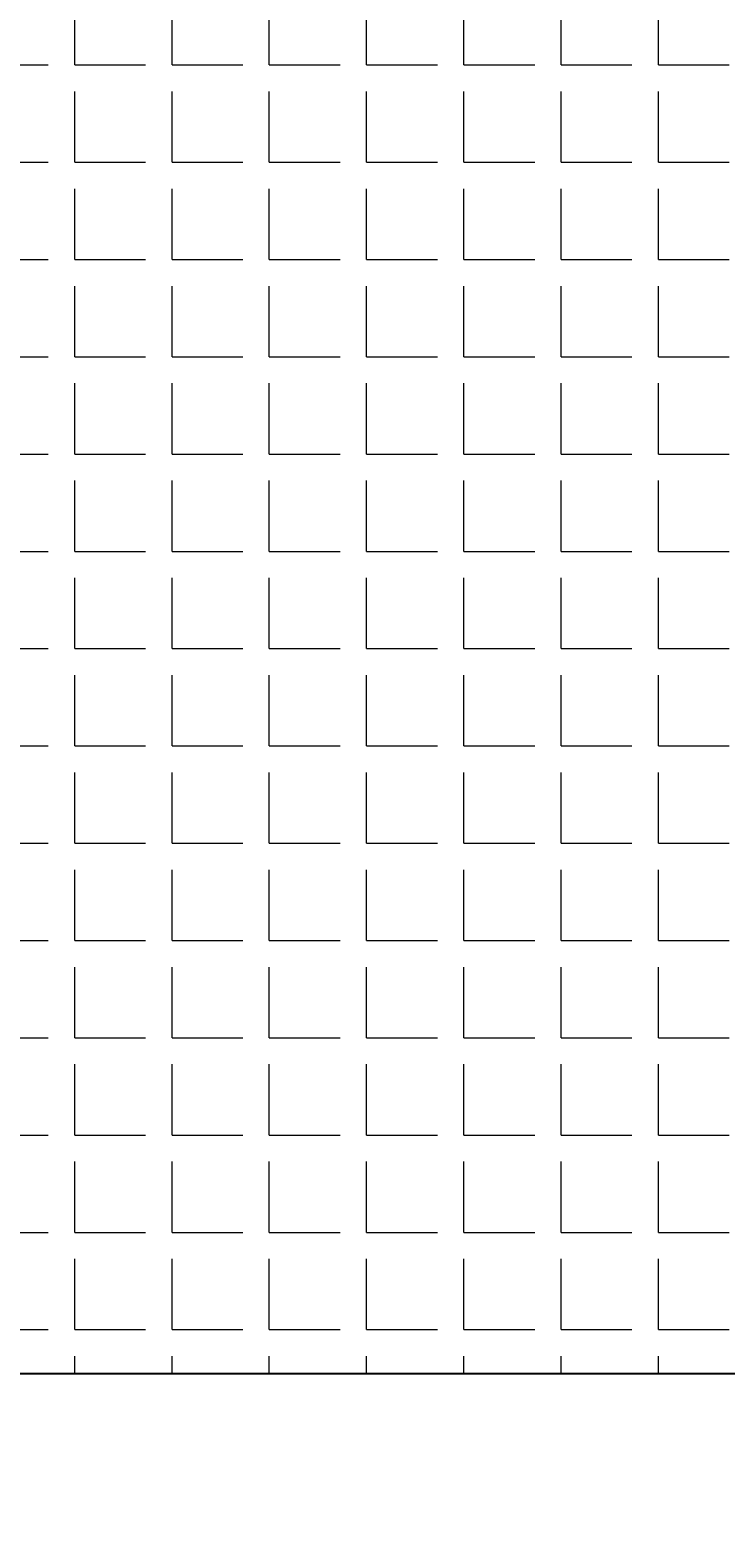
# Model space of a CAD drawing. Units: inches. Extents: x 84 to 1044, y -280 to 906.
# Tile 13 of 105: x 521 to 571, y -132 to -25. Entities that reach past the tile are written whole.
import ezdxf

# ---------------------------------------------------------------- set-up
doc = ezdxf.new("R2010")
doc.units = ezdxf.units.IN
doc.layers.add('A-ANNO-DIMS', color=2, linetype='Continuous', lineweight=18)
doc.layers.add('C-PROP', color=7, linetype='Continuous', lineweight=25)
doc.layers.add('L-HRDS-PATT', color=23, linetype='Continuous', lineweight=9, true_color=0xc2877b)
doc.styles.get("Standard").update_dxf_attribs({"font": 'arial.ttf'})
doc.dimstyles.get("Standard").update_dxf_attribs({"dimtxt": 0.18, "dimasz": 0.18, "dimexe": 0.18, "dimexo": 0.0625, "dimgap": 0.09, "dimtad": 0, "dimtih": 1, "dimtoh": 1, "dimdec": 4, "dimzin": 0, "dimdsep": 46, "dimtxsty": 'Standard', "dimcen": 0.09, "dimadec": 0, "dimazin": 0, "dimtfac": 1, "dimtdec": 4, "dimtofl": 0, "dimtmove": 0, "dimatfit": 3, "dimfxl": 1, "dimtolj": 1, "dimtzin": 0, "dimarcsym": 0})

# ---------------------------------------------------------------- blocks, each defined once
blk = doc.blocks.new('*D60')
at = {"layer": 'A-ANNO-DIMS', "color": 0, "lineweight": -2, "transparency": 16777216}
for p, q in [((134.18, -121.94), (134.18, -180.64)), ((992.07, -121.94), (992.07, -180.64)), ((134.36, -180.46), (562.73, -180.46)), ((991.89, -180.46), (563.52, -180.46))]:
    blk.add_line(p, q, dxfattribs=at)
at = {"layer": 'A-ANNO-DIMS', "color": 0, "transparency": 16777216}
for points in [[(134.36, -180.43), (134.36, -180.49), (134.18, -180.46)], [(991.89, -180.43), (991.89, -180.49), (992.07, -180.46)]]:
    blk.add_solid(points, dxfattribs=at)
at = {"layer": 'Defpoints', "color": 0, "transparency": 16777216}
for p in [(134.18, -121.88), (992.07, -121.88), (992.07, -180.46)]:
    blk.add_point(p, dxfattribs=at)
at = {"layer": 'A-ANNO-DIMS', "color": 0, "transparency": 16777216, "insert": (563.13, -180.46), "char_height": 0.18, "attachment_point": 5}
blk.add_mtext('\\A1;857.9', dxfattribs=at)

msp = doc.modelspace()

# ---------------------------------------------------------------- hatches: boundary and pattern name
at = {"layer": 'L-HRDS-PATT', "transparency": 33554567}
h = msp.add_hatch(dxfattribs=at)
h.set_pattern_fill('ANGLE', color=256)
h.set_pattern_definition([(0, (0, 0), (0, 6.985), [5.08, -1.905]), (90, (0, 0), (-6.985, 4e-16), [5.08, -1.905])])
h.paths.add_polyline_path([(650.074, 31.12), (504.574, 31.12), (504.574, -112.88), (504.574, -121.88), (624.574, -121.88), (624.574, -112.88), (650.074, -112.88)])

# ---------------------------------------------------------------- linework, layer by layer
at = {"layer": 'C-PROP'}
msp.add_line((504.574, -121.88), (624.574, -121.88), dxfattribs=at)

# ---------------------------------------------------------------- dimensions: what is measured, and where the dimension line sits
at = {"layer": 'A-ANNO-DIMS'}
dim = msp.add_linear_dim(base=(992.074, -180.46), p1=(134.179, -121.88), p2=(992.074, -121.88), dimstyle='Standard', override={"dimdec": 1, "dimlfac": 1, "dimrnd": 0, "dimzin": 0, "dimdsep": 46, "dimlunit": 2}, dxfattribs=at)
dim.commit()
dim.dimension.update_dxf_attribs({"geometry": '*D60', "text_midpoint": (563.127, -180.46)})

doc.saveas('drawing.dxf')
